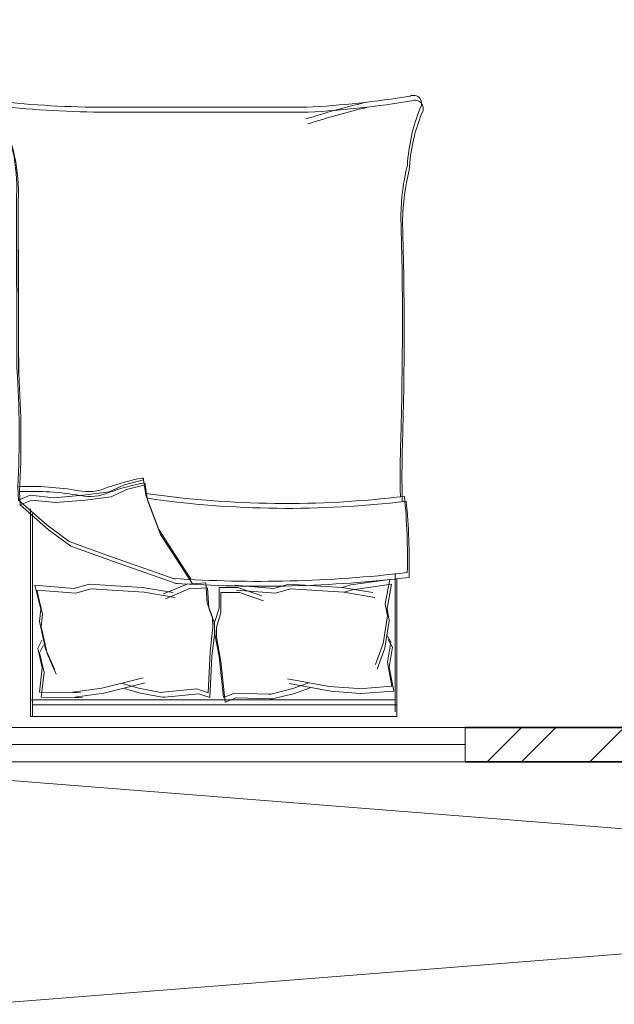
# Model space of a CAD drawing. Units: inches. Extents: x 1885 to 2748, y 783 to 2421.
# Tile 64 of 117: x 2049 to 2127, y 1850 to 1979. Entities that reach past the tile are written whole.
import ezdxf

# ---------------------------------------------------------------- set-up
doc = ezdxf.new("R2010")
doc.units = ezdxf.units.IN
for name, color, linetype, lineweight in [('A-FLOR-OPEN', 8, 'Continuous', 13), ('A-FURN', 8, 'Continuous', 13), ('A-GLAZ', 181, 'Continuous', 18), ('A-WALL', 7, 'Continuous', 35)]:
    doc.layers.add(name, color=color, linetype=linetype, lineweight=lineweight)
doc.layers.add('A-WALL-PATT', color=85, linetype='Continuous', lineweight=13, true_color=0x58ba48)

# ---------------------------------------------------------------- blocks, each defined once
blk = doc.blocks.new('BED-DOUBLE')
for p, q in [((28.39, 53.09), (25.14, 49.39)), ((28.39, 53.09), (25.14, 49.39)), ((29.49, 52.95), (27.75, 52.87, 3.87)), ((29.49, 52.95), (27.75, 52.87, 3.87)), ((30.13, 53.17), (28.39, 53.09, 3.87)), ((30.13, 53.17), (28.39, 53.09, 3.87)), ((29.01, 51.56), (28.39, 53.09)), ((29.01, 51.56), (28.39, 53.09)), ((27.75, 52.87), (24.5, 49.16)), ((27.75, 52.87), (24.5, 49.16)), ((28.37, 51.33), (27.75, 52.87)), ((28.37, 51.33), (27.75, 52.87)), ((0, 51.49), (0.64, 51.49)), ((0, 3.47), (0, 51.49)), ((0, 51.26), (26.61, 51.26)), ((0, 51.26), (26.61, 51.26)), ((0.64, 51.49), (27.25, 51.49)), ((0.64, 51.49), (27.25, 51.49)), ((1.54, 3.47), (1.54, 51.26)), ((1.54, 3.47), (1.54, 51.26)), ((2.18, 3.7), (2.18, 51.49)), ((2.18, 3.7), (2.18, 51.49)), ((6.41, 49.96), (8.98, 50.56)), ((6.41, 49.96), (8.98, 50.56)), ((8.98, 50.56), (10.03, 50.04)), ((8.98, 50.56), (10.03, 50.04)), ((16.58, 50.7), (13.44, 49.92)), ((16.58, 50.7), (13.44, 49.92)), ((17.22, 50.93), (14.08, 50.15)), ((17.22, 50.93), (14.08, 50.15)), ((16.17, 45.57), (16.58, 50.7)), ((16.17, 45.56), (16.58, 50.7)), ((16.81, 45.79), (17.22, 50.93)), ((16.81, 45.79), (17.22, 50.93)), ((28.06, 48.23), (28.37, 51.33)), ((28.06, 48.23), (28.37, 51.33)), ((28.7, 48.46), (29.01, 51.56)), ((28.7, 48.46), (29.01, 51.56)), ((2.56, 50.11), (2.46, 44.71)), ((2.56, 50.11), (2.46, 44.71)), ((2.56, 50.11), (5.77, 49.73)), ((2.56, 50.11), (5.77, 49.73)), ((3.2, 50.34), (3.1, 44.94)), ((3.2, 50.34), (3.1, 44.94)), ((3.2, 50.34), (6.41, 49.96)), ((3.2, 50.34), (6.41, 49.96)), ((8.26, 49.31), (5.58, 48.13)), ((8.26, 49.31), (5.58, 48.13)), ((5.77, 49.73), (8.34, 50.33)), ((5.77, 49.73), (8.34, 50.33)), ((8.9, 49.54), (6.22, 48.36)), ((8.9, 49.54), (6.22, 48.36)), ((11.83, 50.11), (8.26, 49.31)), ((11.83, 50.11), (8.26, 49.31)), ((8.34, 50.33), (9.39, 49.81)), ((8.34, 50.33), (9.39, 49.81)), ((12.47, 50.34), (8.9, 49.54)), ((12.47, 50.34), (8.9, 49.54)), ((13.44, 49.92), (11.83, 50.11)), ((13.44, 49.92), (11.83, 50.11)), ((14.08, 50.15), (12.47, 50.34)), ((14.08, 50.15), (12.47, 50.34)), ((24.5, 49.16), (22.33, 46.22)), ((24.5, 49.16), (22.33, 46.22)), ((25.14, 49.39), (22.97, 46.45)), ((25.14, 49.39), (22.97, 46.45)), ((28.37, 44.36), (28.06, 48.23)), ((28.37, 44.36), (28.06, 48.23)), ((29.01, 44.59), (28.7, 48.46)), ((29.01, 44.59), (28.7, 48.46)), ((2.46, 44.71), (2.55, 45.71)), ((2.46, 44.71), (2.55, 45.71)), ((2.55, 45.71), (3.07, 41.91)), ((2.55, 45.71), (3.07, 41.91)), ((3.1, 44.94), (3.19, 45.94)), ((3.1, 44.94), (3.19, 45.94)), ((3.19, 45.94), (3.71, 42.14)), ((3.19, 45.94), (3.71, 42.14)), ((16.73, 43.6), (16.17, 45.57)), ((16.73, 43.6), (16.17, 45.56)), ((17.37, 43.83), (16.81, 45.79)), ((17.37, 43.83), (16.81, 45.79)), ((22.33, 46.22), (20.32, 40.64)), ((22.33, 46.22), (20.32, 40.64)), ((22.97, 46.45), (20.96, 40.87)), ((22.97, 46.45), (20.96, 40.87)), ((28.83, 40.95), (28.37, 44.36)), ((28.83, 40.95), (28.37, 44.36)), ((29.47, 41.18), (29.01, 44.59)), ((29.47, 41.18), (29.01, 44.59)), ((16.3, 36.59), (16.73, 43.6)), ((16.3, 36.59), (16.73, 43.6)), ((16.94, 36.82), (17.37, 43.83)), ((16.94, 36.82), (17.37, 43.83)), ((3.07, 41.91), (4.43, 36.49)), ((3.07, 41.91), (4.43, 36.49)), ((3.71, 42.14), (5.07, 36.72)), ((3.71, 42.14), (5.07, 36.72)), ((20.32, 40.64), (17.39, 32.3)), ((20.32, 40.64), (17.39, 32.3)), ((20.96, 40.87), (18.03, 32.53)), ((20.96, 40.87), (18.03, 32.53)), ((29.76, 38.94), (28.83, 40.95)), ((29.76, 38.94), (28.83, 40.95)), ((30.4, 39.17), (29.47, 41.18)), ((30.4, 39.17), (29.47, 41.18)), ((3.68, 39.2), (3.08, 37.13)), ((3.68, 39.2), (3.08, 37.13)), ((4.32, 39.43), (3.72, 37.36)), ((4.32, 39.43), (3.72, 37.36)), ((30.38, 36.46), (29.76, 38.94)), ((30.38, 36.46), (29.76, 38.94)), ((31.02, 36.69), (30.4, 39.17)), ((31.02, 36.69), (30.4, 39.17)), ((79.25, 15.06), (79.25, 39.68)), ((79.25, 15.06), (79.25, 39.68)), ((79.89, 15.29), (79.89, 39.9)), ((79.89, 15.29), (79.89, 39.9)), ((3.08, 37.13), (2.54, 34.2)), ((3.08, 37.13), (2.54, 34.2)), ((3.72, 37.36), (3.18, 34.43)), ((3.72, 37.36), (3.18, 34.43)), ((15.63, 32.56), (16.3, 36.59)), ((15.63, 32.56), (16.3, 36.59)), ((16.27, 32.79), (16.94, 36.82)), ((16.27, 32.79), (16.94, 36.82)), ((23.88, 34.45), (28.37, 36.15)), ((23.88, 34.45), (28.37, 36.15)), ((24.52, 34.68), (29.01, 36.38)), ((24.52, 34.68), (29.01, 36.38)), ((28.37, 36.15), (30.38, 36.46)), ((28.37, 36.15), (30.38, 36.46)), ((29.01, 36.38), (31.02, 36.69)), ((29.01, 36.38), (31.02, 36.69)), ((2.54, 34.2), (2.56, 33.88)), ((2.54, 34.2), (2.56, 33.88)), ((2.56, 33.88), (2.98, 29.45)), ((2.56, 33.88), (2.98, 29.45)), ((3.18, 34.43), (3.2, 34.11)), ((3.18, 34.43), (3.2, 34.11)), ((3.2, 34.11), (3.62, 29.68)), ((3.2, 34.11), (3.62, 29.68)), ((16.74, 30.75), (15.46, 33.82)), ((16.74, 30.75), (15.46, 33.82)), ((17.38, 30.98), (16.1, 34.05)), ((17.38, 30.98), (16.1, 34.05)), ((17.39, 30.26), (23.88, 34.45)), ((17.39, 30.26), (23.88, 34.45)), ((18.03, 30.49), (24.52, 34.68)), ((18.03, 30.49), (24.52, 34.68)), ((16.9, 28.3), (16.74, 30.75)), ((16.9, 28.3), (16.74, 30.75)), ((17.54, 28.52), (17.38, 30.98)), ((17.54, 28.52), (17.38, 30.98)), ((2.98, 29.45), (2.5, 27.98)), ((2.98, 29.45), (2.5, 27.98)), ((3.62, 29.68), (3.13, 28.2)), ((3.62, 29.68), (3.13, 28.2)), ((14.86, 28.36), (17.54, 28.52)), ((14.86, 28.36), (17.54, 28.52)), ((2.5, 27.98), (7.87, 27.73)), ((2.5, 27.98), (7.87, 27.73)), ((3.13, 28.2), (8.51, 27.96)), ((3.13, 28.2), (8.51, 27.96)), ((7.22, 26.56), (10.4, 27.14)), ((7.22, 26.56), (10.4, 27.14)), ((7.86, 26.79), (11.04, 27.37)), ((7.86, 26.79), (11.04, 27.37)), ((7.87, 27.73), (11.08, 27.35)), ((7.87, 27.73), (11.08, 27.35)), ((8.51, 27.96), (11.72, 27.58)), ((8.51, 27.96), (11.72, 27.58)), ((10.4, 27.14), (11.71, 27.14)), ((10.4, 27.14), (11.71, 27.14)), ((11.04, 27.37), (12.35, 27.37)), ((11.04, 27.37), (12.35, 27.37)), ((11.08, 27.35), (12.38, 27.43)), ((11.08, 27.35), (12.38, 27.43)), ((11.71, 27.14), (13.59, 26.56)), ((11.71, 27.14), (13.59, 26.56)), ((11.72, 27.58), (13.02, 27.66)), ((11.72, 27.58), (13.02, 27.66)), ((12.35, 27.37), (14.22, 26.79)), ((12.35, 27.37), (14.22, 26.79)), ((12.38, 27.43), (14.22, 28.13)), ((12.38, 27.43), (14.22, 28.13)), ((13.02, 27.66), (14.86, 28.36)), ((13.02, 27.66), (14.86, 28.36)), ((14.22, 28.13), (16.9, 28.3)), ((14.22, 28.13), (16.9, 28.3)), ((1.87, 25.98), (7.22, 26.56)), ((1.87, 25.98), (7.22, 26.56)), ((2.45, 24.54), (1.87, 25.98)), ((2.45, 24.54), (1.87, 25.98)), ((2.51, 26.21), (7.86, 26.79)), ((2.51, 26.21), (7.86, 26.79)), ((3.09, 24.76), (2.51, 26.21)), ((3.09, 24.76), (2.51, 26.21)), ((13.59, 26.56), (16.27, 26.56)), ((13.59, 26.56), (16.27, 26.56)), ((14.22, 26.79), (16.91, 26.79)), ((14.22, 26.79), (16.91, 26.79)), ((16.27, 26.56), (16.27, 24.1)), ((16.27, 26.56), (16.27, 24.1)), ((16.91, 26.79), (16.91, 24.33)), ((16.91, 26.79), (16.91, 24.33)), ((2.31, 20.09), (2.45, 24.54)), ((2.31, 20.09), (2.45, 24.54)), ((2.95, 20.32), (3.09, 24.76)), ((2.95, 20.32), (3.09, 24.76)), ((16.81, 19.61), (17.22, 24.74)), ((16.81, 19.61), (17.22, 24.74)), ((16.27, 24.1), (15.18, 20.96)), ((16.27, 24.1), (15.18, 20.96)), ((16.91, 24.33), (15.82, 21.19)), ((16.91, 24.33), (15.82, 21.19)), ((16.17, 19.38), (16.58, 24.51)), ((16.17, 19.38), (16.58, 24.51)), ((2.31, 19.77), (2.31, 20.09)), ((2.31, 19.77), (2.31, 20.09)), ((3.03, 16.88), (2.31, 19.77)), ((3.03, 16.88), (2.31, 19.77)), ((2.95, 20), (2.95, 20.32)), ((2.95, 20), (2.95, 20.32)), ((3.67, 17.11), (2.95, 20)), ((3.67, 17.11), (2.95, 20)), ((16.73, 17.42), (16.17, 19.38)), ((16.73, 17.42), (16.17, 19.38)), ((17.37, 17.65), (16.81, 19.61)), ((17.37, 17.65), (16.81, 19.61)), ((3.75, 14.85), (3.03, 16.88)), ((3.75, 14.85), (3.03, 16.88)), ((3.32, 12.11), (4.33, 17.6)), ((3.32, 12.11), (4.33, 17.6)), ((4.39, 15.08), (3.67, 17.11)), ((4.39, 15.08), (3.67, 17.11)), ((3.96, 12.34), (4.97, 17.83)), ((3.96, 12.34), (4.97, 17.83)), ((16.3, 10.41), (16.73, 17.42)), ((16.3, 10.41), (16.73, 17.42)), ((16.94, 10.64), (17.37, 17.65)), ((16.94, 10.64), (17.37, 17.65)), ((3.03, 8.28), (3.32, 12.11)), ((3.03, 8.28), (3.32, 12.11)), ((3.67, 8.51), (3.96, 12.34)), ((3.67, 8.51), (3.96, 12.34)), ((15.63, 6.38), (16.3, 10.41)), ((15.63, 6.38), (16.3, 10.41)), ((16.27, 6.61), (16.94, 10.64)), ((16.27, 6.61), (16.94, 10.64)), ((16.3, 10.41), (16.62, 9.28)), ((16.3, 10.41), (16.62, 9.28)), ((16.94, 10.64), (17.26, 9.51)), ((16.94, 10.64), (17.26, 9.51)), ((16.62, 9.28), (17.34, 4.18)), ((16.62, 9.28), (17.34, 4.18)), ((17.26, 9.51), (17.98, 4.41)), ((17.26, 9.51), (17.98, 4.41)), ((3.01, 8.18), (3.03, 8.28)), ((3.01, 8.18), (3.03, 8.28)), ((3.34, 3.9), (3.01, 8.18)), ((3.34, 3.9), (3.01, 8.18)), ((3.65, 8.41), (3.67, 8.51)), ((3.65, 8.41), (3.67, 8.51)), ((3.98, 4.13), (3.65, 8.41)), ((3.98, 4.13), (3.65, 8.41)), ((8.96, 5.05), (6.21, 6.06)), ((8.96, 5.05), (6.21, 6.06)), ((9.6, 5.28), (6.85, 6.29)), ((9.6, 5.28), (6.85, 6.29)), ((13.21, 4.7), (9.6, 5.28)), ((13.21, 4.7), (9.6, 5.28)), ((3.32, 3.89), (6.5, 4.47)), ((3.32, 3.89), (6.5, 4.47)), ((3.96, 4.12), (7.14, 4.7)), ((3.96, 4.12), (7.14, 4.7)), ((6.5, 4.47), (9.1, 4.04)), ((6.5, 4.47), (9.1, 4.04)), ((7.14, 4.7), (9.74, 4.27)), ((7.14, 4.7), (9.74, 4.27)), ((12.57, 4.47), (8.96, 5.05)), ((12.57, 4.47), (8.96, 5.05)), ((9.1, 4.04), (10.12, 4.62)), ((9.1, 4.04), (10.12, 4.62)), ((9.74, 4.27), (10.75, 4.84)), ((9.74, 4.27), (10.75, 4.84)), ((14.16, 4.76), (12.57, 4.47)), ((14.16, 4.76), (12.57, 4.47)), ((14.8, 4.99), (13.21, 4.7)), ((14.8, 4.99), (13.21, 4.7)), ((17.34, 4.18), (14.16, 4.76)), ((17.34, 4.18), (14.16, 4.76)), ((17.98, 4.41), (14.8, 4.99)), ((17.98, 4.41), (14.8, 4.99)), ((18.11, 3.47), (0, 3.47)), ((18.11, 3.47), (0, 3.47)), ((18.75, 3.7), (0.64, 3.7)), ((18.75, 3.7), (0.64, 3.7))]:
    blk.add_line(p, q)
for centre, radius, start, end in [((68.67, 76.16), 23.07, 267.4714, 296.4681), ((68.67, 76.16), 23.07, 267.4714, 296.4681), ((69.31, 76.38), 23.07, 267.4714, 296.4681), ((69.31, 76.38), 23.07, 267.4714, 296.4681), ((78.87, 54.41), 1.1, 332.6588, 86.02), ((78.87, 54.41), 1.1, 332.6588, 86.02), ((79.51, 54.64), 1.1, 332.6588, 86.02), ((79.51, 54.64), 1.1, 332.6588, 86.02), ((-6.65, 51.33), 36.18, 349.8763, 2.5657), ((-6.65, 51.33), 36.18, 349.8763, 2.5657), ((36.32, 182.26), 129.5, 266.9791, 273.8365), ((36.32, 182.26), 129.5, 266.9791, 273.8365), ((-6.01, 51.55), 36.18, 349.8763, 2.5657), ((-6.01, 51.55), 36.18, 349.8763, 2.5657), ((36.96, 182.49), 129.5, 266.9791, 273.8365), ((36.96, 182.49), 129.5, 266.9791, 273.8365), ((67.83, -4508.74), 4561.86, 90.00217, 90.28689), ((67.83, -4508.75), 4561.86, 90.00217, 90.28689), ((68.46, -4508.52), 4561.86, 90.00217, 90.28689), ((68.46, -4508.52), 4561.86, 90.00217, 90.28689), ((212.28, 41.15), 133.04, 174.4998, 180.6351), ((212.28, 41.15), 133.04, 174.4998, 180.6351), ((212.92, 41.38), 133.04, 174.4998, 180.6351), ((212.92, 41.38), 133.04, 174.4998, 180.6351), ((35.71, 43.97), 6.22, 168.6608, 203.7384), ((35.71, 43.97), 6.22, 168.6608, 203.7384), ((35.07, 43.74), 6.22, 168.6608, 203.7384), ((35.07, 43.74), 6.22, 168.6608, 203.7384), ((2.13, 31.38), 29.65, 10.6617, 19.8806), ((2.13, 31.38), 29.65, 10.6617, 19.8806), ((1.49, 31.15), 29.65, 10.6617, 19.8806), ((1.49, 31.15), 29.65, 10.6617, 19.8806), ((156.32, 17.75), 129.02, 171.7845, 186.9006), ((156.32, 17.75), 129.02, 171.7845, 186.9006), ((156.96, 17.98), 129.02, 171.7845, 186.9006), ((156.96, 17.98), 129.02, 171.7845, 186.9006), ((30.44, 36.64), 0.185, 250.2464, 1.1377), ((30.44, 36.63), 0.185, 250.2464, 1.1377), ((31.08, 36.86), 0.185, 250.2464, 1.1377), ((31.08, 36.86), 0.185, 250.2464, 1.1377), ((182.06, 21.36), 164.97, 176.0865, 186.7821), ((182.06, 21.36), 164.97, 176.0865, 186.7821), ((182.7, 21.59), 164.97, 176.0865, 186.7821), ((182.7, 21.59), 164.97, 176.0865, 186.7821), ((-23.71, -17.22), 106.46, 13.3832, 17.7053), ((-23.71, -17.22), 106.46, 13.3832, 17.7053), ((-23.07, -16.99), 106.46, 13.3832, 17.7053), ((-23.07, -16.99), 106.46, 13.3832, 17.7053), ((200.84, 21.43), 121.76, 182.9958, 189.4091), ((200.84, 21.43), 121.76, 182.9958, 189.4091), ((201.48, 21.65), 121.76, 182.9958, 189.4091), ((201.48, 21.65), 121.76, 182.9958, 189.4091), ((31.18, -167.31), 170.11, 88.4762, 91.0082), ((31.18, -167.31), 170.11, 88.4762, 91.0082), ((31.82, -167.08), 170.11, 88.4762, 91.0082), ((31.82, -167.08), 170.11, 88.4762, 91.0082), ((50.62, 484.82), 482.31, 268.2277, 271.7185), ((50.62, 484.82), 482.31, 268.2277, 271.7185), ((51.26, 485.05), 482.31, 268.2277, 271.7185), ((51.26, 485.05), 482.31, 268.2277, 271.7185), ((64.52, -26.9), 29.63, 76.0648, 88.9113), ((64.52, -26.9), 29.63, 76.0648, 88.9113), ((65.16, -26.67), 29.63, 76.0648, 88.9113), ((65.16, -26.67), 29.63, 76.0648, 88.9113), ((20.1, 85.16), 83.31, 268.7218, 275.604), ((20.1, 85.16), 83.31, 268.7218, 275.604), ((20.74, 85.39), 83.31, 268.7218, 275.604), ((20.74, 85.39), 83.31, 268.7218, 275.604), ((70.28, -21.66), 23.56, 67.9751, 86.652), ((70.28, -21.66), 23.56, 67.9751, 86.652), ((70.92, -21.43), 23.56, 67.9751, 86.652), ((70.92, -21.43), 23.56, 67.9751, 86.652), ((79.72, 1.09), 1.09, 236.1736, 23.4781), ((79.72, 1.09), 1.09, 236.1736, 23.4781), ((80.36, 1.31), 1.09, 236.1736, 23.4781), ((80.36, 1.31), 1.09, 236.1736, 23.4781)]:
    blk.add_arc(centre, radius, start, end)
blk = doc.blocks.new('WIN-60')
for p, q in [((0, 60), (4.5, 60)), ((0, 60), (0, 0)), ((4.5, 60), (2.25, 60)), ((2.25, 60), (2.25, 0)), ((4.5, 0), (4.5, 60)), ((2.25, 0), (0, 0)), ((0, 0), (4.5, 0))]:
    blk.add_line(p, q)

msp = doc.modelspace()

# ---------------------------------------------------------------- hatches: boundary and pattern name
at = {"layer": 'A-WALL-PATT'}
h = msp.add_hatch(dxfattribs=at)
h.set_pattern_fill('ANSI32', color=256)
h.paths.add_polyline_path([(2007.77, 2318.01), (1980.77, 2318.01), (1980.77, 2281.22), (1985.27, 2281.22), (1985.27, 2313.51), (2007.77, 2313.51), (2007.77, 2315.76)])
h.paths.add_polyline_path([(2094.32, 2318.01), (2067.77, 2318.01), (2067.77, 2313.51), (2094.32, 2313.51), (2094.32, 2315.76)])
h.paths.add_polyline_path([(2131.37, 2315.76), (2131.37, 2318.01), (2131.19, 2318.01), (2112.61, 2318.01), (2112.61, 2313.51), (2117.27, 2313.51), (2117.27, 2255.2), (2121.77, 2255.2), (2121.77, 2313.51), (2131.37, 2313.51)])
h.paths.add_polyline_path([(2190.51, 2318.01), (2155.37, 2318.01), (2155.37, 2313.51), (2169.77, 2313.51), (2169.77, 2229.51), (2121.77, 2229.51), (2121.77, 2233.45), (2119.52, 2233.45), (2117.27, 2233.45), (2117.27, 2201.1), (2121.77, 2201.1), (2121.77, 2225.01), (2169.77, 2225.01), (2169.77, 2165.01), (2306.27, 2165.01), (2306.27, 2066.01), (2310.77, 2066.01), (2344.27, 2066.01), (2486.27, 2066.01), (2486.27, 1886.01), (2483.02, 1886.01), (2483.02, 1881.51), (2486.27, 1881.51), (2486.27, 1880.68), (2490.77, 1880.68), (2490.77, 2070.51), (2344.27, 2070.51), (2310.77, 2070.51), (2310.77, 2165.01), (2310.77, 2173.64), (2308.52, 2173.64), (2306.27, 2173.64), (2306.27, 2169.51), (2174.27, 2169.51), (2174.27, 2313.51), (2190.51, 2313.51), (2190.51, 2315.76)])
h.paths.add_polyline_path([(1985.27, 2221.22), (1980.77, 2221.22), (1980.77, 2165.01), (1992.77, 2165.01), (1992.77, 2141.93), (1997.27, 2141.93), (1997.27, 2165.01), (2117.27, 2165.01), (2117.27, 2163.13), (2121.77, 2163.13), (2121.77, 2172.73), (2119.52, 2172.73), (2117.27, 2172.73), (2117.27, 2169.51), (1985.27, 2169.51)])
h.paths.add_polyline_path([(1997.27, 2105.93), (1992.77, 2105.93), (1992.77, 2070.51), (2016.77, 2070.51), (2016.77, 2059.12), (2019.02, 2059.12), (2021.27, 2059.12), (2021.27, 2070.51), (2117.27, 2070.51), (2117.27, 2022.51), (2114.42, 2022.51), (2114.42, 2018.01), (2123.63, 2018.01), (2123.63, 2020.26), (2123.63, 2022.51), (2121.77, 2022.51), (2121.77, 2142.59), (2119.52, 2142.59), (2117.27, 2142.59), (2117.27, 2075.01), (1997.27, 2075.01)])
h.paths.add_polyline_path([(2092.03, 2020.26), (2092.03, 2022.51), (2021.27, 2022.51), (2021.27, 2035.12), (2016.77, 2035.12), (2016.77, 2018.01), (2016.77, 1978.78), (2021.27, 1978.78), (2021.27, 2018.01), (2092.03, 2018.01)])
h.paths.add_polyline_path([(2260.94, 2022.51), (2153.1, 2022.51), (2153.1, 2020.26), (2153.1, 2018.01), (2155.27, 2018.01), (2155.27, 1886.01), (2107.63, 1886.01), (2107.63, 1881.51), (2182.91, 1881.51), (2182.91, 1883.76), (2182.91, 1886.01), (2159.77, 1886.01), (2159.77, 2018.01), (2260.94, 2018.01), (2260.94, 2020.26)])
h.paths.add_polyline_path([(2047.63, 1883.76), (2047.63, 1886.01), (2021.27, 1886.01), (2021.27, 1918.78), (2019.02, 1918.78), (2016.77, 1918.78), (2016.77, 1881.51), (2047.63, 1881.51)])
h.paths.add_polyline_path([(2306.36, 1883.76), (2306.36, 1886.01), (2296.27, 1886.01), (2296.27, 1982.01), (2316.54, 1982.01), (2316.54, 1984.26), (2316.54, 1986.51), (2296.27, 1986.51), (2296.27, 2022.51), (2289.28, 2022.51), (2289.28, 2018.01), (2291.77, 2018.01), (2291.77, 1886.01), (2242.91, 1886.01), (2242.91, 1881.51), (2306.36, 1881.51)], flags=17)
h.paths.add_polyline_path([(1985.27, 1843.01), (2021.6, 1843.01), (2021.53, 1845.44), (2021.48, 1847.51), (1980.77, 1847.51), (1980.77, 1809.45), (1985.27, 1809.45)])
h.paths.add_polyline_path([(2131.48, 1845.26), (2131.48, 1847.51), (2081.53, 1847.51), (2081.53, 1843.01), (2117.27, 1843.01), (2117.27, 1784.15), (2119.52, 1784.15), (2121.77, 1784.15), (2121.77, 1843.01), (2131.48, 1843.01)])
h.paths.add_polyline_path([(2203.89, 1847.51), (2155.48, 1847.51), (2155.48, 1843.01), (2169.77, 1843.01), (2169.77, 1759.01), (2121.77, 1759.01), (2121.77, 1761.46), (2117.27, 1761.46), (2117.27, 1730.43), (2121.77, 1730.43), (2121.77, 1754.51), (2177.42, 1754.51), (2177.42, 1756.76), (2177.42, 1759.01), (2174.27, 1759.01), (2174.27, 1843.01), (2203.89, 1843.01)])
h.paths.add_polyline_path([(2335.55, 1845.26), (2335.55, 1847.51), (2239.89, 1847.51), (2239.89, 1843.01), (2306.27, 1843.01), (2306.27, 1759.01), (2199.49, 1759.01), (2199.49, 1754.51), (2310.77, 1754.51), (2310.77, 1843.01), (2335.55, 1843.01)])
h.paths.add_polyline_path([(2348.77, 2022.51), (2344.27, 2022.51), (2344.27, 1986.51), (2341.68, 1986.51), (2341.68, 1982.01), (2344.27, 1982.01), (2344.27, 1886.01), (2330.36, 1886.01), (2330.36, 1881.51), (2361.63, 1881.51), (2361.63, 1883.76), (2361.63, 1886.01), (2348.77, 1886.01)], flags=17)
h.paths.add_polyline_path([(2283.25, 2315.76), (2283.25, 2318.01), (2238.51, 2318.01), (2238.51, 2313.51), (2283.25, 2313.51)], flags=17)
h.paths.add_polyline_path([(2363.27, 2348.01), (2388.68, 2348.01), (2388.68, 2350.26), (2388.68, 2352.51), (2358.77, 2352.51), (2358.77, 2348.01), (2358.77, 2318.01), (2344.48, 2318.01), (2344.48, 2313.51), (2358.77, 2313.51), (2358.77, 2229.51), (2310.77, 2229.51), (2310.77, 2231.95), (2306.27, 2231.95), (2306.27, 2205.61), (2310.77, 2205.61), (2310.77, 2225.01), (2358.77, 2225.01), (2358.77, 2211.51), (2452.33, 2211.51), (2452.33, 2213.76), (2452.33, 2216.01), (2363.27, 2216.01), (2363.27, 2318.01)])
h.paths.add_polyline_path([(2310.77, 2313.51), (2320.48, 2313.51), (2320.48, 2315.76), (2320.48, 2318.01), (2302.73, 2318.01), (2302.73, 2313.51), (2306.27, 2313.51), (2306.27, 2251.08), (2310.77, 2251.08)], flags=17)
h.paths.add_polyline_path([(2490.77, 2352.51), (2486.27, 2352.51), (2448.68, 2352.51), (2448.68, 2348.01), (2486.27, 2348.01), (2486.27, 2318.01), (2486.27, 2216.01), (2481.78, 2216.01), (2481.78, 2211.51), (2486.27, 2211.51), (2486.27, 2165.01), (2493.29, 2165.01), (2493.29, 2167.26), (2493.29, 2169.51), (2490.77, 2169.51), (2490.77, 2313.51), (2494.43, 2313.51), (2494.43, 2318.01), (2490.77, 2318.01)])
h.paths.add_polyline_path([(2534.65, 2318.01), (2515.69, 2318.01), (2515.69, 2313.51), (2534.65, 2313.51), (2534.65, 2315.76)])
h.paths.add_polyline_path([(2618.27, 2318.01), (2594.65, 2318.01), (2594.65, 2313.51), (2613.77, 2313.51), (2613.77, 2281.71), (2618.27, 2281.71)])
h.paths.add_polyline_path([(2618.27, 2221.71), (2613.77, 2221.71), (2613.77, 2169.51), (2554.02, 2169.51), (2554.02, 2165.01), (2613.77, 2165.01), (2613.77, 2152.88), (2618.27, 2152.88)])
h.paths.add_polyline_path([(2618.27, 2128.88), (2616.02, 2128.88), (2613.77, 2128.88), (2613.77, 2117.01), (2529.77, 2117.01), (2529.77, 2165.01), (2532.85, 2165.01), (2532.85, 2169.51), (2522.87, 2169.51), (2522.87, 2165.01), (2525.27, 2165.01), (2525.27, 2117.01), (2525.27, 2112.51), (2525.27, 2108.58), (2529.77, 2108.58), (2529.77, 2112.51), (2613.77, 2112.51), (2613.77, 2080.19), (2618.27, 2080.19)])
h.paths.add_polyline_path([(2618.27, 2044.19), (2616.02, 2044.19), (2613.77, 2044.19), (2613.77, 2015.51), (2529.77, 2015.51), (2529.77, 2088.58), (2527.52, 2088.58), (2525.27, 2088.58), (2525.27, 2011.01), (2613.77, 2011.01), (2613.77, 1956.75), (2618.27, 1956.75)])
h.paths.add_polyline_path([(2618.27, 1881.51), (2618.27, 1896.75), (2613.77, 1896.75), (2613.77, 1881.51), (2613.77, 1847.51), (2592.71, 1847.51), (2592.71, 1843.01), (2613.77, 1843.01), (2613.77, 1765.01), (2613.77, 1760.51), (2609.62, 1760.51), (2609.62, 1756.01), (2613.77, 1756.01), (2613.77, 1660.01), (2608.54, 1660.01), (2608.54, 1655.51), (2613.77, 1655.51), (2613.77, 1508.16), (2618.27, 1508.16)])
h.paths.add_polyline_path([(2565.77, 1843.01), (2569, 1843.01), (2569, 1847.51), (2490.77, 1847.51), (2490.77, 1849.7), (2488.52, 1849.7), (2486.27, 1849.7), (2486.27, 1847.51), (2477.27, 1847.51), (2477.27, 1838.51), (2477.27, 1821.49), (2486.27, 1821.49), (2486.27, 1838.51), (2561.27, 1838.51), (2561.27, 1765.01), (2486.27, 1765.01), (2486.27, 1786.16), (2477.27, 1786.16), (2477.27, 1765.01), (2477.27, 1756.01), (2486.27, 1756.01), (2565.77, 1756.01), (2585.62, 1756.01), (2585.62, 1758.26), (2585.62, 1760.51), (2565.77, 1760.51), (2565.77, 1765.01)])
h.paths.add_polyline_path([(2486.27, 1651.01), (2561.27, 1651.01), (2561.27, 1567.01), (2486.27, 1567.01), (2486.27, 1591.32), (2477.27, 1591.32), (2477.27, 1567.01), (2477.27, 1558.01), (2477.27, 1555.44), (2481.77, 1555.44), (2481.77, 1558.01), (2568.65, 1558.01), (2568.65, 1560.26), (2568.65, 1562.51), (2565.77, 1562.51), (2565.77, 1655.51), (2584.54, 1655.51), (2584.54, 1657.76), (2584.54, 1660.01), (2565.77, 1660.01), (2486.27, 1660.01), (2477.27, 1660.01), (2477.27, 1651.01), (2477.27, 1632.99), (2486.27, 1632.99)])
h.paths.add_polyline_path([(2449.97, 1883.76), (2449.97, 1886.01), (2421.63, 1886.01), (2421.63, 1881.51), (2449.97, 1881.51)], flags=17)
h.paths.add_polyline_path([(2447.27, 1847.51), (2395.55, 1847.51), (2395.55, 1843.01), (2442.77, 1843.01), (2442.77, 1809.27), (2447.27, 1809.27)])
h.paths.add_polyline_path([(1985.27, 1749.45), (1980.77, 1749.45), (1980.77, 1694.5), (1985.27, 1694.5), (1985.27, 1694.51), (1986.9, 1694.51), (1986.9, 1697.78), (1986.9, 1699.01), (1985.27, 1699.01)])
h.paths.add_polyline_path([(2152.77, 1699.01), (2121.77, 1699.01), (2121.77, 1703.67), (2119.52, 1703.67), (2117.27, 1703.67), (2117.27, 1699.01), (2009.22, 1699.01), (2009.22, 1694.51), (2148.27, 1694.51), (2148.27, 1692.63), (2152.77, 1692.63)])
h.paths.add_polyline_path([(2016.27, 1694.51), (2011.77, 1694.51), (2011.77, 1558.01), (2040.81, 1558.01), (2040.81, 1560.26), (2040.81, 1562.51), (2016.27, 1562.51)])
h.paths.add_polyline_path([(2152.77, 1663.02), (2150.52, 1663.02), (2148.27, 1663.02), (2148.27, 1562.51), (2100.81, 1562.51), (2100.81, 1558.01), (2165.12, 1558.01), (2165.12, 1560.26), (2165.12, 1562.51), (2152.77, 1562.51), (2152.77, 1610.51), (2224.77, 1610.51), (2224.77, 1607.99), (2229.27, 1607.99), (2229.27, 1615.01), (2152.77, 1615.01)])
h.paths.add_polyline_path([(2238.61, 1560.26), (2238.61, 1562.51), (2229.27, 1562.51), (2229.27, 1588.76), (2227.02, 1588.76), (2224.77, 1588.77), (2224.77, 1562.51), (2189.12, 1562.51), (2189.12, 1558.01), (2238.61, 1558.01)])
h.paths.add_polyline_path([(2336.02, 1560.26), (2336.02, 1562.51), (2310.77, 1562.51), (2310.77, 1656.35), (2308.52, 1656.35), (2306.27, 1656.35), (2306.27, 1562.51), (2286.61, 1562.51), (2286.61, 1558.01), (2336.02, 1558.01)])
h.paths.add_polyline_path([(2447.27, 1690.97), (2445.02, 1690.97), (2442.77, 1690.97), (2442.77, 1687.01), (2306.27, 1687.01), (2306.27, 1680.75), (2310.77, 1680.75), (2310.77, 1682.51), (2442.77, 1682.51), (2442.77, 1562.51), (2396.02, 1562.51), (2396.02, 1558.01), (2447.27, 1558.01)])
h.paths.add_polyline_path([(2447.27, 1749.27), (2445.02, 1749.27), (2442.77, 1749.27), (2442.77, 1717.23), (2447.27, 1717.23)])
h.paths.add_polyline_path([(2044.67, 1521.76), (2044.67, 1524.01), (2007.27, 1524.01), (2007.27, 1503.49), (2009.52, 1503.49), (2011.77, 1503.49), (2011.77, 1519.51), (2044.67, 1519.51)])
h.paths.add_polyline_path([(2177.97, 1521.76), (2177.97, 1524.01), (2104.67, 1524.01), (2104.67, 1519.51), (2145.77, 1519.51), (2145.77, 1387.51), (2143.37, 1387.51), (2143.37, 1383.01), (2251.59, 1383.01), (2251.59, 1385.26), (2251.59, 1387.51), (2150.27, 1387.51), (2150.27, 1519.51), (2177.97, 1519.51)])
h.paths.add_polyline_path([(2298.7, 1524.01), (2237.97, 1524.01), (2237.97, 1519.51), (2282.27, 1519.51), (2282.27, 1387.51), (2279.68, 1387.51), (2279.68, 1383.01), (2286.77, 1383.01), (2286.77, 1419.01), (2312.45, 1419.01), (2312.45, 1421.26), (2312.45, 1423.51), (2286.77, 1423.51), (2286.77, 1519.51), (2298.7, 1519.51), (2298.7, 1521.72)], flags=17)
h.paths.add_polyline_path([(2361.9, 1521.76), (2361.9, 1524.01), (2322.7, 1524.01), (2322.7, 1519.51), (2334.77, 1519.51), (2334.77, 1423.51), (2331.93, 1423.51), (2331.93, 1419.01), (2334.77, 1419.01), (2334.77, 1387.51), (2334.77, 1383.23), (2339.27, 1383.23), (2339.27, 1387.51), (2339.27, 1519.51), (2361.9, 1519.51)], flags=17)
h.paths.add_polyline_path([(2447.27, 1521.76), (2447.27, 1524.01), (2421.9, 1524.01), (2421.9, 1519.51), (2447.27, 1519.51)], flags=17)
h.paths.add_polyline_path([(2481.77, 1529.6), (2479.52, 1529.6), (2477.27, 1529.6), (2477.27, 1524.01), (2474.49, 1524.01), (2474.49, 1519.51), (2477.27, 1519.51), (2477.27, 1334.51), (2296.77, 1334.51), (2296.77, 1240.51), (2160.27, 1240.51), (2160.27, 1180.51), (2112.27, 1180.51), (2112.27, 1207.69), (2110.02, 1207.69), (2107.77, 1207.69), (2107.77, 1171.61), (2112.27, 1171.61), (2112.27, 1176.01), (2160.27, 1176.01), (2160.27, 1092.01), (2144.22, 1092.01), (2144.22, 1087.51), (2189.5, 1087.51), (2189.5, 1089.76), (2189.5, 1092.01), (2164.77, 1092.01), (2164.77, 1236.01), (2296.77, 1236.01), (2296.77, 1231.91), (2301.27, 1231.91), (2301.27, 1330.01), (2481.77, 1330.01), (2481.77, 1387.51)])
h.paths.add_polyline_path([(2618.27, 1448.16), (2613.77, 1448.16), (2613.77, 1382.51), (2529.77, 1382.51), (2525.27, 1382.51), (2525.27, 1307.06), (2529.77, 1307.06), (2529.77, 1378.01), (2613.77, 1378.01), (2613.77, 1354.99), (2618.27, 1354.99)])
h.paths.add_polyline_path([(2618.27, 1318.99), (2613.77, 1318.99), (2613.77, 1281.01), (2529.77, 1281.01), (2529.77, 1283.79), (2527.52, 1283.79), (2525.27, 1283.79), (2525.27, 1228.51), (2516.79, 1228.51), (2516.79, 1224.01), (2533.48, 1224.01), (2533.48, 1226.26), (2533.48, 1228.51), (2529.77, 1228.51), (2529.77, 1276.51), (2613.77, 1276.51), (2613.77, 1266.02), (2618.27, 1266.02)])
h.paths.add_polyline_path([(2618.27, 1134.96), (2613.77, 1134.96), (2613.77, 1092.01), (2594.54, 1092.01), (2594.54, 1087.51), (2618.27, 1087.51)])
h.paths.add_polyline_path([(2534.54, 1092.01), (2509.77, 1092.01), (2509.77, 1087.51), (2534.54, 1087.51), (2534.54, 1089.76)])
h.paths.add_polyline_path([(2481.27, 1224.01), (2484.12, 1224.01), (2484.12, 1226.26), (2484.12, 1228.51), (2476.77, 1228.51), (2476.77, 1198.51), (2471.61, 1198.51), (2471.61, 1194.01), (2476.77, 1194.01), (2476.77, 1062.01), (2436.89, 1062.01), (2436.89, 1057.51), (2476.77, 1057.51), (2481.27, 1057.51), (2481.27, 1062.01), (2481.27, 1087.51), (2485.35, 1087.51), (2485.35, 1089.76), (2485.35, 1092.01), (2481.27, 1092.01), (2481.27, 1117.51)])
h.paths.add_polyline_path([(2439.9, 1198.51), (2349.27, 1198.51), (2349.27, 1194.01), (2349.27, 1180.51), (2301.27, 1180.51), (2301.27, 1201.9), (2299.02, 1201.9), (2296.77, 1201.9), (2296.77, 1172.34), (2299.02, 1172.34), (2301.27, 1172.34), (2301.27, 1176.01), (2349.27, 1176.01), (2349.27, 1092.01), (2334.45, 1092.01), (2334.45, 1087.51), (2349.27, 1087.51), (2349.27, 1057.51), (2353.77, 1057.51), (2376.89, 1057.51), (2376.89, 1059.76), (2376.89, 1062.01), (2353.77, 1062.01), (2353.77, 1087.51), (2353.77, 1180.51), (2353.77, 1194.01), (2439.9, 1194.01), (2439.9, 1196.26)])
h.paths.add_polyline_path([(2270.6, 1089.76), (2270.6, 1092.01), (2249.5, 1092.01), (2249.5, 1087.51), (2270.6, 1087.51)], flags=17)
h.paths.add_polyline_path([(2310.45, 1092.01), (2301.27, 1092.01), (2301.27, 1153.29), (2296.77, 1153.29), (2296.77, 1092.01), (2293.79, 1092.01), (2293.79, 1087.51), (2310.45, 1087.51), (2310.45, 1089.76)], flags=17)
h.paths.add_polyline_path([(2112.27, 1150.33), (2110.02, 1150.33), (2107.77, 1150.33), (2107.77, 1092.01), (2104.47, 1092.01), (2104.47, 1087.51), (2120.22, 1087.51), (2120.22, 1089.76), (2120.22, 1092.01), (2112.27, 1092.01)])
h.paths.add_polyline_path([(2082.17, 1092.01), (2058.14, 1092.01), (2058.14, 1087.51), (2082.17, 1087.51), (2082.17, 1089.76)])
h.paths.add_polyline_path([(1975.77, 1145.64), (1971.27, 1145.64), (1971.27, 1087.51), (1980.77, 1087.51), (1998.14, 1087.51), (1998.14, 1089.76), (1998.14, 1092.01), (1985.27, 1092.01), (1975.77, 1092.01)])
h.paths.add_polyline_path([(2112.27, 1244.38), (2110.02, 1244.38), (2107.77, 1244.38), (2107.77, 1240.51), (1992.27, 1240.51), (1992.27, 1271.01), (1987.77, 1271.01), (1987.77, 1240.51), (1980.77, 1240.51), (1975.77, 1240.51), (1971.27, 1240.51), (1971.27, 1205.64), (1975.77, 1205.64), (1975.77, 1236.01), (2107.77, 1236.01), (2107.77, 1233.44), (2112.27, 1233.44), (2112.27, 1236.01)])
h.paths.add_polyline_path([(2112.27, 1383.01), (2114.78, 1383.01), (2114.78, 1385.26), (2114.78, 1387.51), (2102.48, 1387.51), (2102.48, 1383.01), (2107.77, 1383.01), (2107.77, 1335.01), (2011.77, 1335.01), (2011.77, 1349.94), (2007.27, 1349.94), (2007.27, 1335.01), (1987.77, 1335.01), (1987.77, 1330.51), (1987.77, 1307.01), (1992.27, 1307.01), (1992.27, 1330.51), (2007.27, 1330.51), (2107.77, 1330.51), (2107.77, 1264.71), (2112.27, 1264.71)])
h.paths.add_polyline_path([(2077.86, 1387.51), (2011.77, 1387.51), (2011.77, 1390.04), (2009.52, 1390.04), (2007.27, 1390.04), (2007.27, 1373.94), (2011.77, 1373.94), (2011.77, 1383.01), (2077.86, 1383.01)])
h.paths.add_polyline_path([(2011.77, 1443.49), (2007.27, 1443.49), (2007.27, 1410.25), (2011.77, 1410.25)])

# ---------------------------------------------------------------- linework, layer by layer
at = {"layer": 'A-FLOR-OPEN'}
for p, q in [((2016.77, 1847.51), (2447.27, 1881.51)), ((2447.27, 1847.51), (2016.77, 1881.51))]:
    msp.add_line(p, q, dxfattribs=at)
at = {"layer": 'A-WALL'}
for p, q in [((2107.63, 1886.01), (2155.27, 1886.01)), ((2107.63, 1881.51), (2182.91, 1881.51)), ((2107.63, 1881.51), (2117.27, 1881.51))]:
    msp.add_line(p, q, dxfattribs=at)

# ---------------------------------------------------------------- block references
at = {"layer": 'A-FURN', "rotation": 89.9999998331857}
msp.add_blockref('BED-DOUBLE', (2102.14, 1887.42), dxfattribs=at)
at = {"layer": 'A-GLAZ', "extrusion": (0, 0, -1), "zscale": -1, "rotation": 90}
msp.add_blockref('WIN-60', (-2047.63, 1881.5), dxfattribs=at)

doc.saveas('drawing.dxf')
